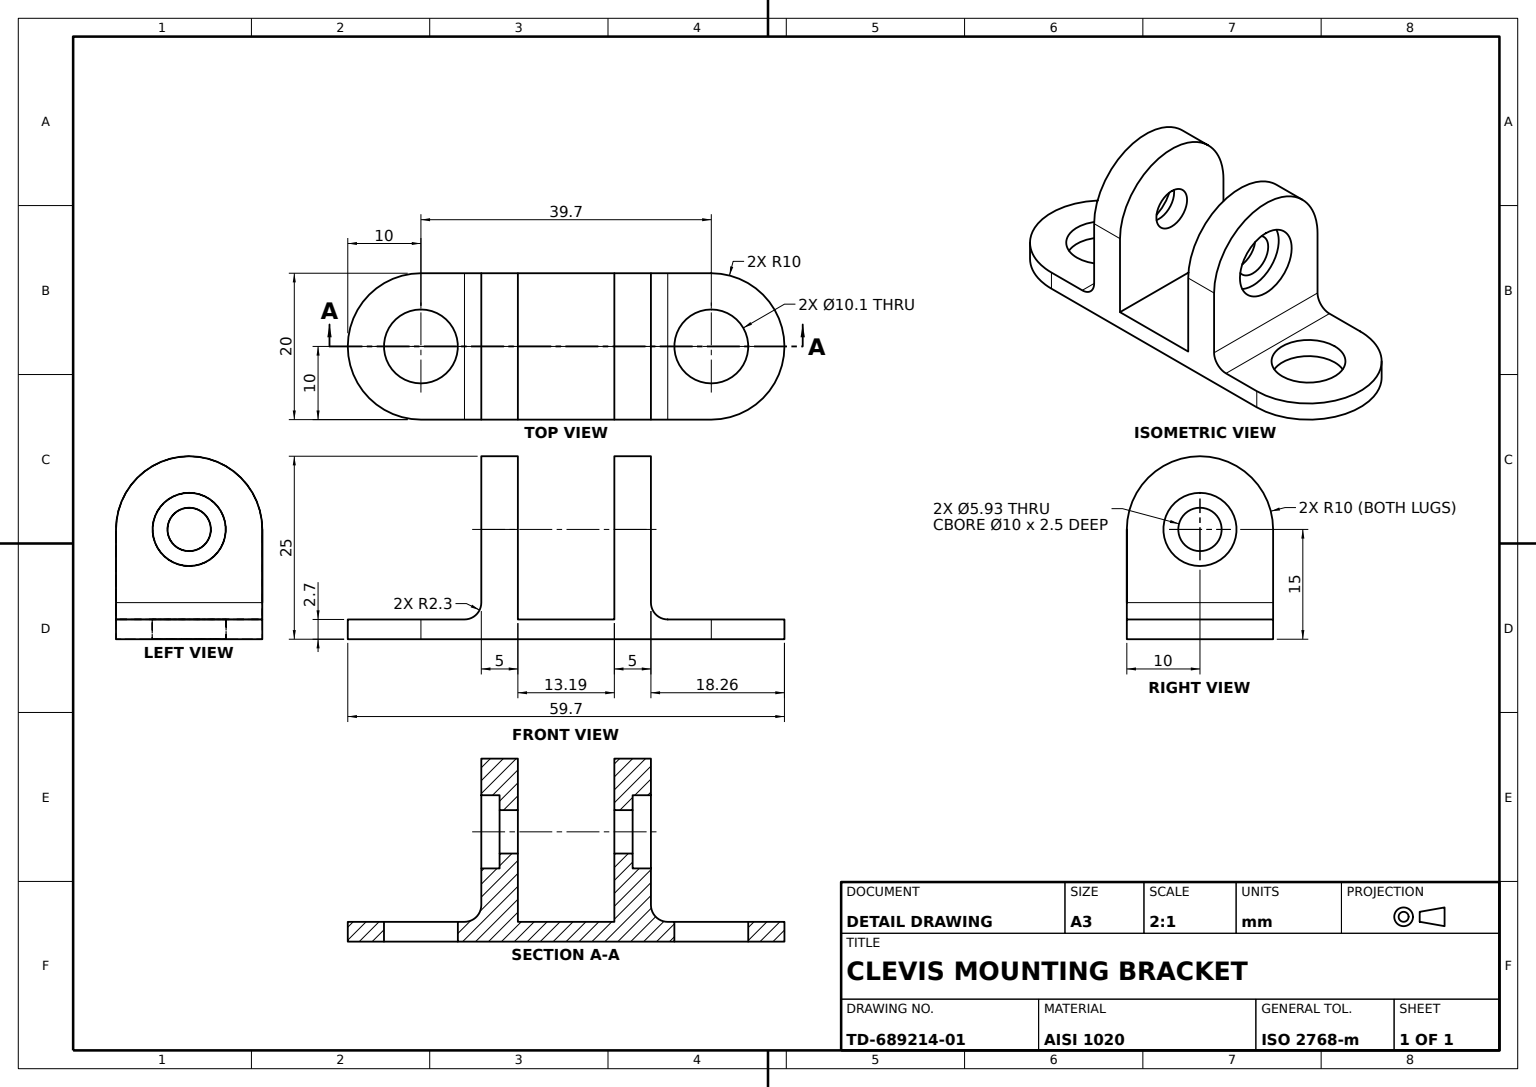
SolidWorks part; units mm, degrees
material "AISI 1020"
ref_plane "Front Plane" through (0, 0, 0) normal (0, 0, 1) x (1, 0, 0)
ref_plane "Top Plane" through (0, 0, 0) normal (0, 1, 0) x (1, 0, 0)
ref_plane "Right Plane" through (0, 0, 0) normal (1, 0, 0) x (0, 0, -1)
sketch "Base Plate Sketch" plane through (0, 0, 0) normal (0, 1, 0) x (1, 0, 0)
  line L0 (-19.85, 0) -> (19.85, 0) construction
  line L1 (-19.85, 10) -> (19.85, 10)
  line L2 (-19.85, -10) -> (19.85, -10)
  arc A0 (-19.85, 10) -> (-19.85, -10) centre (-19.85, 0) ccw
  arc A1 (19.85, -10) -> (19.85, 10) centre (19.85, 0) ccw
  circle A2 centre (-19.85, 0) radius 5.05
  circle A3 centre (19.85, 0) radius 5.05
  point P2 (0, 0)
  dimension "D2" = 10
  dimension "D3" = 10.1
  dimension "D1" = 39.7
extrude "Base Plate" add sketch "Base Plate Sketch" along normal blind 2.7
sketch "Lug Sketch" plane through (0, 0, 10) normal (0, 0, 1) x (1, 0, 0)
  line L0 (0, 0) -> (0, 23.2567) construction
  line L1 (-6.595, 2.7) -> (-6.595, 15)
  line L2 (-19.85, 2.7) -> (19.85, 2.7) construction
  line L3 (-6.595, 15) -> (-11.595, 15)
  line L4 (-11.595, 15) -> (-11.595, 2.7)
  line L5 (-11.595, 2.7) -> (-6.595, 2.7)
  line L6 (-19.85, 0) -> (19.85, 0) construction
  dimension "D1" = 5
  dimension "D2" = 6.595
  dimension "D3" = 15
extrude "Lug" add sketch "Lug Sketch" against normal up to surface (20 mm away) up to face at (0, 1.35, -10)
sketch "Lug Web Sketch" plane through (-11.595, 0, 0) normal (-1, 0, 0) x (0, 0, 1)
  line L0 (-10, 15) -> (10, 15)
  arc A0 (-10, 15) -> (10, 15) centre (0, 15) cw
  dimension "D1" = 10
extrude "Lug Web" add sketch "Lug Web Sketch" against normal up to surface (5 mm away) up to face at (-6.595, 8.85, 0)
mirror "Base Plate Mirror" about plane through (0, 0, 0) normal (1, 0, 0) of bodies 103
fillet "Fillet R2.3" radius 2.3 2 edges at (11.595, 2.7, 0) (-11.595, 2.7, 0)
sketch "Pin Hole Sketch" plane through (-11.595, 0, 0) normal (-1, 0, 0) x (0, 0, 1)
  circle A0 centre (0, 15) radius 2.965
  dimension "D1" = 5.93
extrude "Pin Hole Ø5.93" cut sketch "Pin Hole Sketch" against normal up to surface (5 mm away) up to face at (-6.595, 11.35, 0)
sketch "Counterbore Sketch" plane through (-11.595, 0, 0) normal (-1, 0, 0) x (0, 0, 1)
  circle A0 centre (0, 15) radius 5
  dimension "D1" = 10
extrude "Counterbore Ø10x2.5" cut sketch "Counterbore Sketch" against normal blind 2.5
mirror "Pin Hole Mirror" about plane through (0, 0, 0) normal (1, 0, 0) of "Counterbore Ø10x2.5", "Pin Hole Ø5.93"
